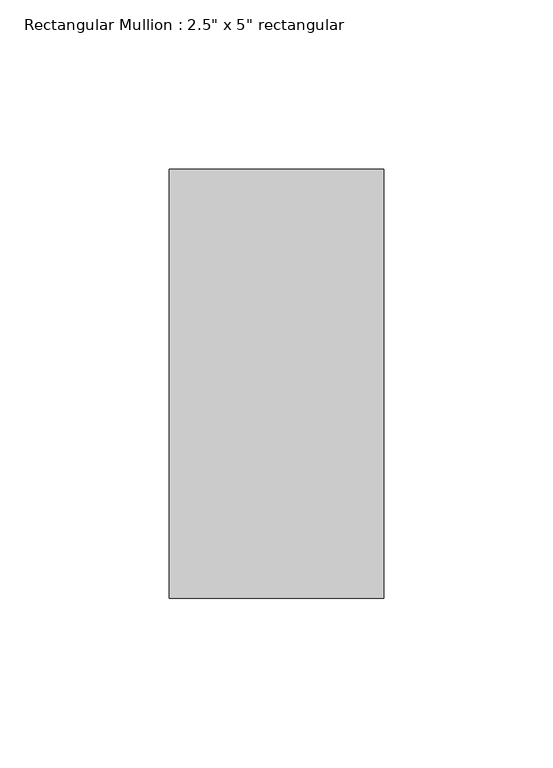
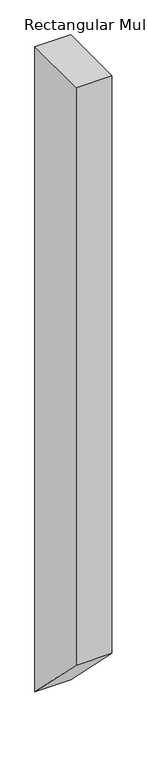
"""IFC4 building model written with IfcOpenShell, lengths in millimetres: member geometry."""

from ifc_helpers import new_model, si_unit, frame, origin, place, context, project, spatial, polyline, outline, extrude, source, transform, mapped, element, save


def member_80100a85(model_context):
    return source(origin(), model_context, "Body", "SweptSolid", [
        extrude(outline(polyline([(-63.5, 0.0), (63.5, 0.0), (63.5, -1217.2950002), (-63.5, -1090.2950002), (-63.5, 0.0)])), frame((-31.75, 0.0, 0.0), z_axis=(1.0, 0.0, 0.0), x_axis=(0.0, 1.0, 0.0)), (0.0, 0.0, 1.0), 63.5),
    ])


if __name__ == "__main__":
    model = new_model("IFC4")
    model_context = context("Model", 3, world=origin())
    ifc_project = project(units=[si_unit("LENGTHUNIT", "METRE", prefix="MILLI")], contexts=[model_context])
    site = spatial("IfcSite", under=ifc_project)
    building = spatial("IfcBuilding", under=site)
    placement = place(None, origin())
    member_shape = member_80100a85(model_context)
    element("IfcMember", 1, ObjectType="Rectangular Mullion : 2.5\" x 5\" rectangular", at=placement, inside=building, context=model_context, shape_type="MappedRepresentation", body=[
        mapped(member_shape, transform((0.0, 0.0, 0.0), x_axis=(1.0, 0.0, 0.0), y_axis=(0.0, 1.0, 0.0), z_axis=(0.0, 0.0, 1.0))),
    ])
    save(model, "model.ifc")

# Revit data of these elements
# Type "Rectangular Mullion : 2.5\" x 5\" rectangular"
#   built-in parameter 1007304 = 0.416667 (stored number, unit not read)
#   built-in parameter 1007301 = 0.104167 (stored number, unit not read)
#   built-in parameter 1007300 = 0.104167 (stored number, unit not read)
# Element 1 (IfcMember, "Rectangular Mullion : 2.5\" x 5\" rectangular")
#   Materials on its faces: "Aluminum"
# Materials
#   "Aluminum": class "Metal", colour RGB 247 247 247, transparency 0, Description = "Aluminum 6061", Cost = 0
